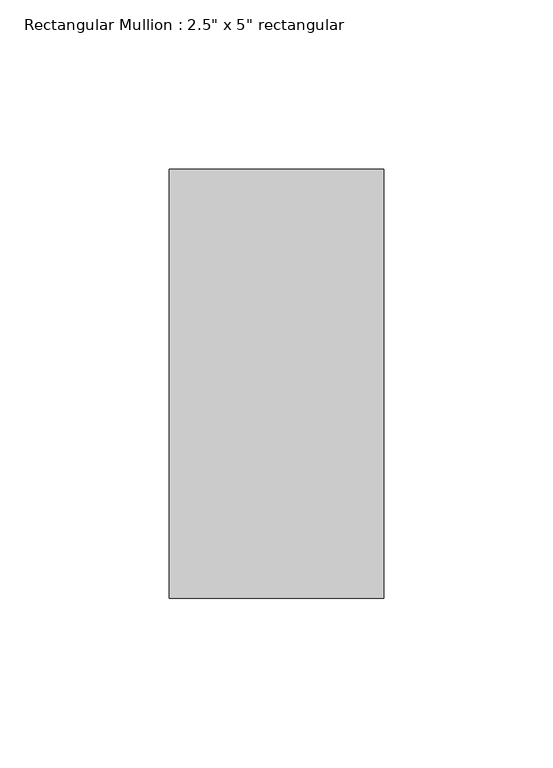
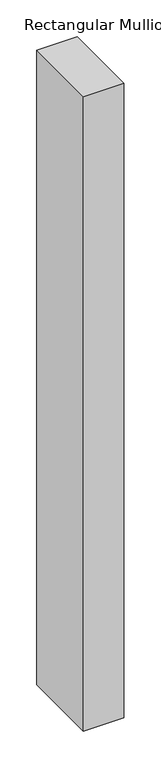
"""IFC4 building model written with IfcOpenShell, lengths in millimetres: member geometry."""

from ifc_helpers import new_model, si_unit, frame, origin, place, context, project, spatial, polyline, outline, extrude, source, transform, mapped, element, save


def member_afdd3af2(model_context):
    return source(origin(), model_context, "Body", "SweptSolid", [
        extrude(outline(polyline([(31.75, 63.5), (31.75, -63.5), (-31.75, -63.5), (-31.75, 63.5), (31.75, 63.5)])), frame((0.0, 0.0, -1054.1), z_axis=(0.0, 0.0, 1.0), x_axis=(1.0, 0.0, 0.0)), (0.0, 0.0, 1.0), 1054.1),
    ])


if __name__ == "__main__":
    model = new_model("IFC4")
    model_context = context("Model", 3, world=origin())
    ifc_project = project(units=[si_unit("LENGTHUNIT", "METRE", prefix="MILLI")], contexts=[model_context])
    site = spatial("IfcSite", under=ifc_project)
    building = spatial("IfcBuilding", under=site)
    placement = place(None, origin())
    member_shape = member_afdd3af2(model_context)
    element("IfcMember", 1, ObjectType="Rectangular Mullion : 2.5\" x 5\" rectangular", at=placement, inside=building, context=model_context, shape_type="MappedRepresentation", body=[
        mapped(member_shape, transform((0.0, 0.0, 0.0), x_axis=(1.0, 0.0, 0.0), y_axis=(0.0, 1.0, 0.0), z_axis=(0.0, 0.0, 1.0))),
    ])
    save(model, "model.ifc")

# Revit data of these elements
# Type "Rectangular Mullion : 2.5\" x 5\" rectangular"
#   built-in parameter 1007304 = 0.416667 (stored number, unit not read)
#   built-in parameter 1007301 = 0.104167 (stored number, unit not read)
#   built-in parameter 1007300 = 0.104167 (stored number, unit not read)
# Element 1 (IfcMember, "Rectangular Mullion : 2.5\" x 5\" rectangular")
#   Materials on its faces: "Aluminum"
# Materials
#   "Aluminum": class "Metal", colour RGB 247 247 247, transparency 0, Description = "Aluminum 6061", Cost = 0
